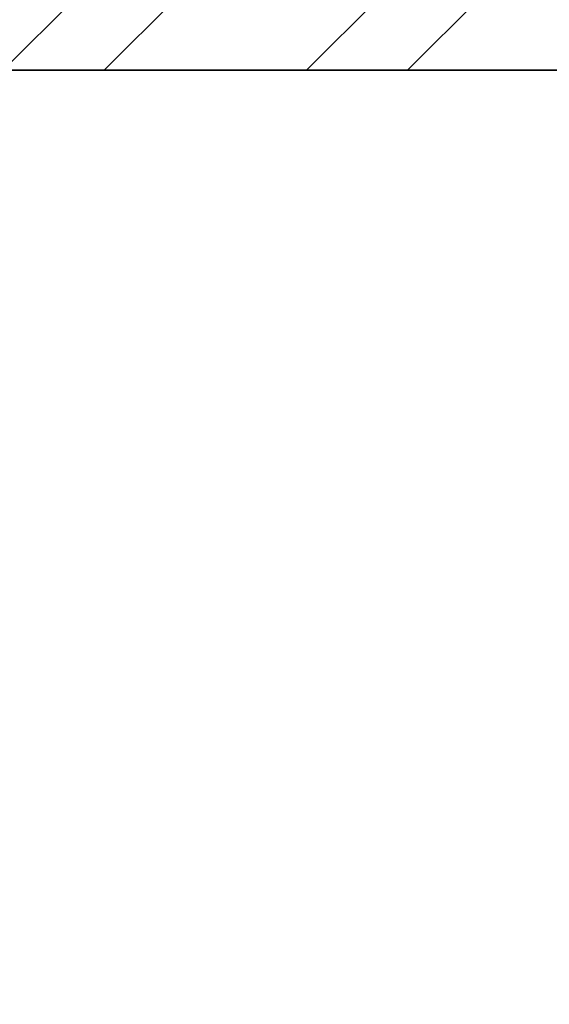
# Model space of a CAD drawing. Units: inches. Extents: x 1885 to 2748, y 783 to 2421.
# Tile 113 of 117: x 2571 to 2595, y 2071 to 2115. Entities that reach past the tile are written whole.
import ezdxf

# ---------------------------------------------------------------- set-up
doc = ezdxf.new("R2010")
doc.units = ezdxf.units.IN
doc.layers.add('A-WALL', color=7, linetype='Continuous', lineweight=35)
doc.layers.add('A-WALL-PATT', color=85, linetype='Continuous', lineweight=13, true_color=0x58ba48)

msp = doc.modelspace()

# ---------------------------------------------------------------- hatches: boundary and pattern name
at = {"layer": 'A-WALL-PATT'}
h = msp.add_hatch(dxfattribs=at)
h.set_pattern_fill('ANSI32', color=256)
h.paths.add_polyline_path([(2007.772, 2318.006), (1980.774, 2318.006), (1980.774, 2281.215), (1985.274, 2281.215), (1985.274, 2313.506), (2007.772, 2313.506), (2007.772, 2315.756)])
h.paths.add_polyline_path([(2094.324, 2318.006), (2067.772, 2318.006), (2067.772, 2313.506), (2094.324, 2313.506), (2094.324, 2315.756)])
h.paths.add_polyline_path([(2131.367, 2315.756), (2131.367, 2318.006), (2131.189, 2318.006), (2112.609, 2318.006), (2112.609, 2313.506), (2117.274, 2313.506), (2117.274, 2255.201), (2121.774, 2255.201), (2121.774, 2313.506), (2131.367, 2313.506)])
h.paths.add_polyline_path([(2190.512, 2318.006), (2155.367, 2318.006), (2155.367, 2313.506), (2169.774, 2313.506), (2169.774, 2229.506), (2121.774, 2229.506), (2121.774, 2233.451), (2119.524, 2233.451), (2117.274, 2233.451), (2117.274, 2201.101), (2121.774, 2201.101), (2121.774, 2225.006), (2169.774, 2225.006), (2169.774, 2165.006), (2306.274, 2165.006), (2306.274, 2066.006), (2310.774, 2066.006), (2344.274, 2066.006), (2486.274, 2066.006), (2486.274, 1886.006), (2483.02, 1886.006), (2483.02, 1881.506), (2486.274, 1881.506), (2486.274, 1880.678), (2490.774, 1880.678), (2490.774, 2070.506), (2344.274, 2070.506), (2310.774, 2070.506), (2310.774, 2165.006), (2310.774, 2173.636), (2308.524, 2173.636), (2306.274, 2173.636), (2306.274, 2169.506), (2174.274, 2169.506), (2174.274, 2313.506), (2190.512, 2313.506), (2190.512, 2315.756)])
h.paths.add_polyline_path([(1985.274, 2221.215), (1980.774, 2221.215), (1980.774, 2165.006), (1992.774, 2165.006), (1992.774, 2141.927), (1997.274, 2141.927), (1997.274, 2165.006), (2117.274, 2165.006), (2117.274, 2163.126), (2121.774, 2163.126), (2121.774, 2172.734), (2119.524, 2172.734), (2117.274, 2172.734), (2117.274, 2169.506), (1985.274, 2169.506)])
h.paths.add_polyline_path([(1997.274, 2105.927), (1992.774, 2105.927), (1992.774, 2070.506), (2016.774, 2070.506), (2016.774, 2059.123), (2019.024, 2059.123), (2021.274, 2059.123), (2021.274, 2070.506), (2117.274, 2070.506), (2117.274, 2022.506), (2114.423, 2022.506), (2114.423, 2018.006), (2123.627, 2018.006), (2123.627, 2020.256), (2123.627, 2022.506), (2121.774, 2022.506), (2121.774, 2142.587), (2119.524, 2142.587), (2117.274, 2142.587), (2117.274, 2075.006), (1997.274, 2075.006)])
h.paths.add_polyline_path([(2092.029, 2020.256), (2092.029, 2022.506), (2021.274, 2022.506), (2021.274, 2035.123), (2016.774, 2035.123), (2016.774, 2018.006), (2016.774, 1978.784), (2021.274, 1978.784), (2021.274, 2018.006), (2092.029, 2018.006)])
h.paths.add_polyline_path([(2260.938, 2022.506), (2153.105, 2022.506), (2153.105, 2020.256), (2153.105, 2018.006), (2155.274, 2018.006), (2155.274, 1886.006), (2107.629, 1886.006), (2107.629, 1881.506), (2182.911, 1881.506), (2182.911, 1883.756), (2182.911, 1886.006), (2159.774, 1886.006), (2159.774, 2018.006), (2260.938, 2018.006), (2260.938, 2020.256)])
h.paths.add_polyline_path([(2047.629, 1883.756), (2047.629, 1886.006), (2021.274, 1886.006), (2021.274, 1918.784), (2019.024, 1918.784), (2016.774, 1918.784), (2016.774, 1881.506), (2047.629, 1881.506)])
h.paths.add_polyline_path([(2306.361, 1883.756), (2306.361, 1886.006), (2296.274, 1886.006), (2296.274, 1982.006), (2316.535, 1982.006), (2316.535, 1984.256), (2316.535, 1986.506), (2296.274, 1986.506), (2296.274, 2022.506), (2289.276, 2022.506), (2289.276, 2018.006), (2291.774, 2018.006), (2291.774, 1886.006), (2242.911, 1886.006), (2242.911, 1881.506), (2306.361, 1881.506)], flags=17)
h.paths.add_polyline_path([(1985.274, 1843.006), (2021.6, 1843.006), (2021.534, 1845.441), (2021.477, 1847.506), (1980.774, 1847.506), (1980.774, 1809.446), (1985.274, 1809.446)])
h.paths.add_polyline_path([(2131.482, 1845.256), (2131.482, 1847.506), (2081.534, 1847.506), (2081.534, 1843.006), (2117.274, 1843.006), (2117.274, 1784.147), (2119.524, 1784.147), (2121.774, 1784.147), (2121.774, 1843.006), (2131.482, 1843.006)])
h.paths.add_polyline_path([(2203.886, 1847.506), (2155.482, 1847.506), (2155.482, 1843.006), (2169.774, 1843.006), (2169.774, 1759.006), (2121.774, 1759.006), (2121.774, 1761.457), (2117.274, 1761.457), (2117.274, 1730.429), (2121.774, 1730.429), (2121.774, 1754.506), (2177.421, 1754.506), (2177.421, 1756.756), (2177.421, 1759.006), (2174.274, 1759.006), (2174.274, 1843.006), (2203.886, 1843.006)])
h.paths.add_polyline_path([(2335.554, 1845.256), (2335.554, 1847.506), (2239.886, 1847.506), (2239.886, 1843.006), (2306.274, 1843.006), (2306.274, 1759.006), (2199.486, 1759.006), (2199.486, 1754.506), (2310.774, 1754.506), (2310.774, 1843.006), (2335.554, 1843.006)])
h.paths.add_polyline_path([(2348.774, 2022.506), (2344.274, 2022.506), (2344.274, 1986.506), (2341.681, 1986.506), (2341.681, 1982.006), (2344.274, 1982.006), (2344.274, 1886.006), (2330.361, 1886.006), (2330.361, 1881.506), (2361.627, 1881.506), (2361.627, 1883.756), (2361.627, 1886.006), (2348.774, 1886.006)], flags=17)
h.paths.add_polyline_path([(2283.251, 2315.756), (2283.251, 2318.006), (2238.512, 2318.006), (2238.512, 2313.506), (2283.251, 2313.506)], flags=17)
h.paths.add_polyline_path([(2363.274, 2348.006), (2388.677, 2348.006), (2388.677, 2350.256), (2388.677, 2352.506), (2358.774, 2352.506), (2358.774, 2348.006), (2358.774, 2318.006), (2344.481, 2318.006), (2344.481, 2313.506), (2358.774, 2313.506), (2358.774, 2229.506), (2310.774, 2229.506), (2310.774, 2231.952), (2306.274, 2231.952), (2306.274, 2205.611), (2310.774, 2205.611), (2310.774, 2225.006), (2358.774, 2225.006), (2358.774, 2211.506), (2452.329, 2211.506), (2452.329, 2213.756), (2452.329, 2216.006), (2363.274, 2216.006), (2363.274, 2318.006)])
h.paths.add_polyline_path([(2310.774, 2313.506), (2320.481, 2313.506), (2320.481, 2315.756), (2320.481, 2318.006), (2302.728, 2318.006), (2302.728, 2313.506), (2306.274, 2313.506), (2306.274, 2251.076), (2310.774, 2251.076)], flags=17)
h.paths.add_polyline_path([(2490.774, 2352.506), (2486.274, 2352.506), (2448.677, 2352.506), (2448.677, 2348.006), (2486.274, 2348.006), (2486.274, 2318.006), (2486.274, 2216.006), (2481.78, 2216.006), (2481.78, 2211.506), (2486.274, 2211.506), (2486.274, 2165.006), (2493.289, 2165.006), (2493.289, 2167.256), (2493.289, 2169.506), (2490.774, 2169.506), (2490.774, 2313.506), (2494.429, 2313.506), (2494.429, 2318.006), (2490.774, 2318.006)])
h.paths.add_polyline_path([(2534.653, 2318.006), (2515.691, 2318.006), (2515.691, 2313.506), (2534.653, 2313.506), (2534.653, 2315.756)])
h.paths.add_polyline_path([(2618.274, 2318.006), (2594.653, 2318.006), (2594.653, 2313.506), (2613.774, 2313.506), (2613.774, 2281.706), (2618.274, 2281.706)])
h.paths.add_polyline_path([(2618.274, 2221.706), (2613.774, 2221.706), (2613.774, 2169.506), (2554.019, 2169.506), (2554.019, 2165.006), (2613.774, 2165.006), (2613.774, 2152.878), (2618.274, 2152.878)])
h.paths.add_polyline_path([(2618.274, 2128.878), (2616.024, 2128.878), (2613.774, 2128.878), (2613.774, 2117.006), (2529.774, 2117.006), (2529.774, 2165.006), (2532.848, 2165.006), (2532.848, 2169.506), (2522.867, 2169.506), (2522.867, 2165.006), (2525.274, 2165.006), (2525.274, 2117.006), (2525.274, 2112.506), (2525.274, 2108.576), (2529.774, 2108.576), (2529.774, 2112.506), (2613.774, 2112.506), (2613.774, 2080.19), (2618.274, 2080.19)])
h.paths.add_polyline_path([(2618.274, 2044.19), (2616.024, 2044.19), (2613.774, 2044.19), (2613.774, 2015.506), (2529.774, 2015.506), (2529.774, 2088.582), (2527.524, 2088.582), (2525.274, 2088.582), (2525.274, 2011.006), (2613.774, 2011.006), (2613.774, 1956.755), (2618.274, 1956.755)])
h.paths.add_polyline_path([(2618.274, 1881.506), (2618.274, 1896.755), (2613.774, 1896.755), (2613.774, 1881.506), (2613.774, 1847.506), (2592.715, 1847.506), (2592.715, 1843.006), (2613.774, 1843.006), (2613.774, 1765.006), (2613.774, 1760.506), (2609.621, 1760.506), (2609.621, 1756.006), (2613.774, 1756.006), (2613.774, 1660.006), (2608.544, 1660.006), (2608.544, 1655.506), (2613.774, 1655.506), (2613.774, 1508.158), (2618.274, 1508.158)])
h.paths.add_polyline_path([(2565.774, 1843.006), (2568.997, 1843.006), (2568.997, 1847.506), (2490.774, 1847.506), (2490.774, 1849.7), (2488.524, 1849.7), (2486.274, 1849.7), (2486.274, 1847.506), (2477.274, 1847.506), (2477.274, 1838.506), (2477.274, 1821.493), (2486.274, 1821.493), (2486.274, 1838.506), (2561.274, 1838.506), (2561.274, 1765.006), (2486.274, 1765.006), (2486.274, 1786.157), (2477.274, 1786.157), (2477.274, 1765.006), (2477.274, 1756.006), (2486.274, 1756.006), (2565.774, 1756.006), (2585.621, 1756.006), (2585.621, 1758.256), (2585.621, 1760.506), (2565.774, 1760.506), (2565.774, 1765.006)])
h.paths.add_polyline_path([(2486.274, 1651.006), (2561.274, 1651.006), (2561.274, 1567.006), (2486.274, 1567.006), (2486.274, 1591.321), (2477.274, 1591.321), (2477.274, 1567.006), (2477.274, 1558.006), (2477.274, 1555.439), (2481.774, 1555.439), (2481.774, 1558.006), (2568.653, 1558.006), (2568.653, 1560.256), (2568.653, 1562.506), (2565.774, 1562.506), (2565.774, 1655.506), (2584.544, 1655.506), (2584.544, 1657.756), (2584.544, 1660.006), (2565.774, 1660.006), (2486.274, 1660.006), (2477.274, 1660.006), (2477.274, 1651.006), (2477.274, 1632.989), (2486.274, 1632.989)])
h.paths.add_polyline_path([(2449.967, 1883.756), (2449.967, 1886.006), (2421.627, 1886.006), (2421.627, 1881.506), (2449.967, 1881.506)], flags=17)
h.paths.add_polyline_path([(2447.274, 1847.506), (2395.554, 1847.506), (2395.554, 1843.006), (2442.774, 1843.006), (2442.774, 1809.27), (2447.274, 1809.27)])
h.paths.add_polyline_path([(1985.274, 1749.446), (1980.774, 1749.446), (1980.774, 1694.504), (1985.274, 1694.504), (1985.274, 1694.506), (1986.897, 1694.506), (1986.897, 1697.78), (1986.897, 1699.006), (1985.274, 1699.006)])
h.paths.add_polyline_path([(2152.774, 1699.006), (2121.774, 1699.006), (2121.774, 1703.668), (2119.524, 1703.668), (2117.274, 1703.668), (2117.274, 1699.006), (2009.219, 1699.006), (2009.219, 1694.506), (2148.274, 1694.506), (2148.274, 1692.631), (2152.774, 1692.631)])
h.paths.add_polyline_path([(2016.274, 1694.506), (2011.774, 1694.506), (2011.774, 1558.006), (2040.806, 1558.006), (2040.806, 1560.256), (2040.806, 1562.506), (2016.274, 1562.506)])
h.paths.add_polyline_path([(2152.774, 1663.017), (2150.524, 1663.017), (2148.274, 1663.017), (2148.274, 1562.506), (2100.806, 1562.506), (2100.806, 1558.006), (2165.119, 1558.006), (2165.119, 1560.256), (2165.119, 1562.506), (2152.774, 1562.506), (2152.774, 1610.506), (2224.774, 1610.506), (2224.774, 1607.99), (2229.274, 1607.99), (2229.274, 1615.006), (2152.774, 1615.006)])
h.paths.add_polyline_path([(2238.613, 1560.256), (2238.613, 1562.506), (2229.274, 1562.506), (2229.274, 1588.756), (2227.024, 1588.763), (2224.774, 1588.771), (2224.774, 1562.506), (2189.119, 1562.506), (2189.119, 1558.006), (2238.613, 1558.006)])
h.paths.add_polyline_path([(2336.024, 1560.256), (2336.024, 1562.506), (2310.774, 1562.506), (2310.774, 1656.347), (2308.524, 1656.347), (2306.274, 1656.347), (2306.274, 1562.506), (2286.613, 1562.506), (2286.613, 1558.006), (2336.024, 1558.006)])
h.paths.add_polyline_path([(2447.274, 1690.968), (2445.024, 1690.968), (2442.774, 1690.968), (2442.774, 1687.006), (2306.274, 1687.006), (2306.274, 1680.75), (2310.774, 1680.75), (2310.774, 1682.506), (2442.774, 1682.506), (2442.774, 1562.506), (2396.024, 1562.506), (2396.024, 1558.006), (2447.274, 1558.006)])
h.paths.add_polyline_path([(2447.274, 1749.27), (2445.024, 1749.27), (2442.774, 1749.27), (2442.774, 1717.232), (2447.274, 1717.232)])
h.paths.add_polyline_path([(2044.674, 1521.756), (2044.674, 1524.006), (2007.274, 1524.006), (2007.274, 1503.49), (2009.524, 1503.49), (2011.774, 1503.49), (2011.774, 1519.506), (2044.674, 1519.506)])
h.paths.add_polyline_path([(2177.969, 1521.756), (2177.969, 1524.006), (2104.674, 1524.006), (2104.674, 1519.506), (2145.774, 1519.506), (2145.774, 1387.506), (2143.37, 1387.506), (2143.37, 1383.006), (2251.585, 1383.006), (2251.585, 1385.256), (2251.585, 1387.506), (2150.274, 1387.506), (2150.274, 1519.506), (2177.969, 1519.506)])
h.paths.add_polyline_path([(2298.704, 1524.006), (2237.969, 1524.006), (2237.969, 1519.506), (2282.274, 1519.506), (2282.274, 1387.506), (2279.683, 1387.506), (2279.683, 1383.006), (2286.774, 1383.006), (2286.774, 1419.006), (2312.451, 1419.006), (2312.451, 1421.256), (2312.451, 1423.506), (2286.774, 1423.506), (2286.774, 1519.506), (2298.704, 1519.506), (2298.704, 1521.722)], flags=17)
h.paths.add_polyline_path([(2361.897, 1521.756), (2361.897, 1524.006), (2322.704, 1524.006), (2322.704, 1519.506), (2334.774, 1519.506), (2334.774, 1423.506), (2331.93, 1423.506), (2331.93, 1419.006), (2334.774, 1419.006), (2334.774, 1387.506), (2334.774, 1383.228), (2339.274, 1383.228), (2339.274, 1387.506), (2339.274, 1519.506), (2361.897, 1519.506)], flags=17)
h.paths.add_polyline_path([(2447.274, 1521.756), (2447.274, 1524.006), (2421.897, 1524.006), (2421.897, 1519.506), (2447.274, 1519.506)], flags=17)
h.paths.add_polyline_path([(2481.774, 1529.6), (2479.524, 1529.6), (2477.274, 1529.6), (2477.274, 1524.006), (2474.489, 1524.006), (2474.489, 1519.506), (2477.274, 1519.506), (2477.274, 1334.506), (2296.774, 1334.506), (2296.774, 1240.506), (2160.274, 1240.506), (2160.274, 1180.506), (2112.274, 1180.506), (2112.274, 1207.692), (2110.024, 1207.692), (2107.774, 1207.692), (2107.774, 1171.609), (2112.274, 1171.609), (2112.274, 1176.006), (2160.274, 1176.006), (2160.274, 1092.006), (2144.221, 1092.006), (2144.221, 1087.506), (2189.497, 1087.506), (2189.497, 1089.756), (2189.497, 1092.006), (2164.774, 1092.006), (2164.774, 1236.006), (2296.774, 1236.006), (2296.774, 1231.912), (2301.274, 1231.912), (2301.274, 1330.006), (2481.774, 1330.006), (2481.774, 1387.506)])
h.paths.add_polyline_path([(2618.274, 1448.158), (2613.774, 1448.158), (2613.774, 1382.506), (2529.774, 1382.506), (2525.274, 1382.506), (2525.274, 1307.062), (2529.774, 1307.062), (2529.774, 1378.006), (2613.774, 1378.006), (2613.774, 1354.988), (2618.274, 1354.988)])
h.paths.add_polyline_path([(2618.274, 1318.988), (2613.774, 1318.988), (2613.774, 1281.006), (2529.774, 1281.006), (2529.774, 1283.786), (2527.524, 1283.786), (2525.274, 1283.786), (2525.274, 1228.506), (2516.794, 1228.506), (2516.794, 1224.006), (2533.484, 1224.006), (2533.484, 1226.256), (2533.484, 1228.506), (2529.774, 1228.506), (2529.774, 1276.506), (2613.774, 1276.506), (2613.774, 1266.02), (2618.274, 1266.02)])
h.paths.add_polyline_path([(2618.274, 1134.964), (2613.774, 1134.964), (2613.774, 1092.006), (2594.545, 1092.006), (2594.545, 1087.506), (2618.274, 1087.506)])
h.paths.add_polyline_path([(2534.545, 1092.006), (2509.765, 1092.006), (2509.765, 1087.506), (2534.545, 1087.506), (2534.545, 1089.756)])
h.paths.add_polyline_path([(2481.274, 1224.006), (2484.117, 1224.006), (2484.117, 1226.256), (2484.117, 1228.506), (2476.774, 1228.506), (2476.774, 1198.506), (2471.61, 1198.506), (2471.61, 1194.006), (2476.774, 1194.006), (2476.774, 1062.006), (2436.894, 1062.006), (2436.894, 1057.506), (2476.774, 1057.506), (2481.274, 1057.506), (2481.274, 1062.006), (2481.274, 1087.506), (2485.354, 1087.506), (2485.354, 1089.756), (2485.354, 1092.006), (2481.274, 1092.006), (2481.274, 1117.506)])
h.paths.add_polyline_path([(2439.898, 1198.506), (2349.274, 1198.506), (2349.274, 1194.006), (2349.274, 1180.506), (2301.274, 1180.506), (2301.274, 1201.896), (2299.024, 1201.896), (2296.774, 1201.896), (2296.774, 1172.335), (2299.024, 1172.335), (2301.274, 1172.335), (2301.274, 1176.006), (2349.274, 1176.006), (2349.274, 1092.006), (2334.452, 1092.006), (2334.452, 1087.506), (2349.274, 1087.506), (2349.274, 1057.506), (2353.774, 1057.506), (2376.894, 1057.506), (2376.894, 1059.756), (2376.894, 1062.006), (2353.774, 1062.006), (2353.774, 1087.506), (2353.774, 1180.506), (2353.774, 1194.006), (2439.898, 1194.006), (2439.898, 1196.256)])
h.paths.add_polyline_path([(2270.596, 1089.756), (2270.596, 1092.006), (2249.497, 1092.006), (2249.497, 1087.506), (2270.596, 1087.506)], flags=17)
h.paths.add_polyline_path([(2310.452, 1092.006), (2301.274, 1092.006), (2301.274, 1153.292), (2296.774, 1153.292), (2296.774, 1092.006), (2293.786, 1092.006), (2293.786, 1087.506), (2310.452, 1087.506), (2310.452, 1089.756)], flags=17)
h.paths.add_polyline_path([(2112.274, 1150.328), (2110.024, 1150.328), (2107.774, 1150.328), (2107.774, 1092.006), (2104.465, 1092.006), (2104.465, 1087.506), (2120.221, 1087.506), (2120.221, 1089.756), (2120.221, 1092.006), (2112.274, 1092.006)])
h.paths.add_polyline_path([(2082.172, 1092.006), (2058.144, 1092.006), (2058.144, 1087.506), (2082.172, 1087.506), (2082.172, 1089.756)])
h.paths.add_polyline_path([(1975.774, 1145.638), (1971.274, 1145.638), (1971.274, 1087.506), (1980.774, 1087.506), (1998.144, 1087.506), (1998.144, 1089.756), (1998.144, 1092.006), (1985.274, 1092.006), (1975.774, 1092.006)])
h.paths.add_polyline_path([(2112.274, 1244.385), (2110.024, 1244.385), (2107.774, 1244.385), (2107.774, 1240.506), (1992.274, 1240.506), (1992.274, 1271.008), (1987.774, 1271.008), (1987.774, 1240.506), (1980.774, 1240.506), (1975.774, 1240.506), (1971.274, 1240.506), (1971.274, 1205.638), (1975.774, 1205.638), (1975.774, 1236.006), (2107.774, 1236.006), (2107.774, 1233.444), (2112.274, 1233.444), (2112.274, 1236.006)])
h.paths.add_polyline_path([(2112.274, 1383.006), (2114.783, 1383.006), (2114.783, 1385.256), (2114.783, 1387.506), (2102.476, 1387.506), (2102.476, 1383.006), (2107.774, 1383.006), (2107.774, 1335.006), (2011.774, 1335.006), (2011.774, 1349.939), (2007.274, 1349.939), (2007.274, 1335.006), (1987.774, 1335.006), (1987.774, 1330.506), (1987.774, 1307.008), (1992.274, 1307.008), (1992.274, 1330.506), (2007.274, 1330.506), (2107.774, 1330.506), (2107.774, 1264.711), (2112.274, 1264.711)])
h.paths.add_polyline_path([(2077.857, 1387.506), (2011.774, 1387.506), (2011.774, 1390.036), (2009.524, 1390.036), (2007.274, 1390.036), (2007.274, 1373.939), (2011.774, 1373.939), (2011.774, 1383.006), (2077.857, 1383.006)])
h.paths.add_polyline_path([(2011.774, 1443.49), (2007.274, 1443.49), (2007.274, 1410.248), (2011.774, 1410.248)])

# ---------------------------------------------------------------- linework, layer by layer
at = {"layer": 'A-WALL'}
msp.add_line((2529.774, 2112.506), (2613.774, 2112.506), dxfattribs=at)

doc.saveas('drawing.dxf')
